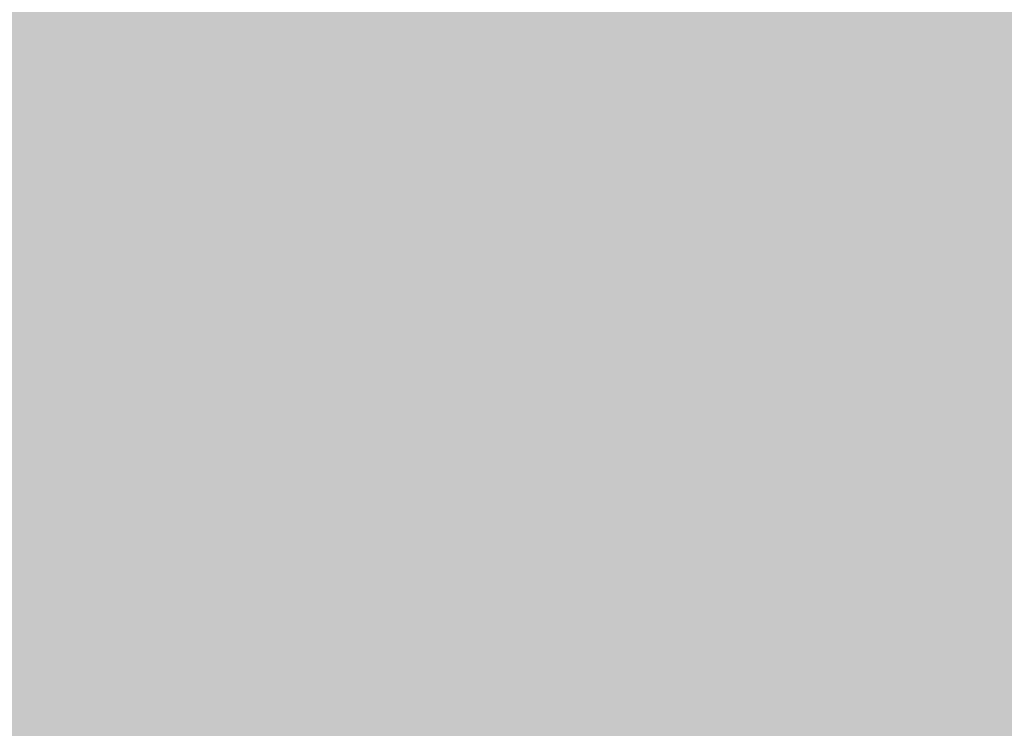
# Model space of a CAD drawing. Units: feet. Extents: x 3168 to 4724, y 827 to 1477.
# Tile 182 of 256: x 3307.378 to 3316.072, y 1087.401 to 1093.654. Entities that reach past the tile are written whole.
import ezdxf

# ---------------------------------------------------------------- set-up
doc = ezdxf.new("R2010")
doc.units = ezdxf.units.FT
doc.layers.add('A-ELEV-PATT', color=8, linetype='Continuous', lineweight=13)

msp = doc.modelspace()

# ---------------------------------------------------------------- hatches: boundary and pattern name
at = {"layer": 'A-ELEV-PATT'}
h = msp.add_hatch(color=256, dxfattribs=at)
h.dxf.hatch_style = 1
edge = h.paths.add_edge_path()
edge.add_ellipse((3552.9058, 979.2201), major_axis=(36.7449, 0), ratio=0.4848485, start_angle=0, end_angle=360)
edge = h.paths.add_edge_path()
edge.add_ellipse((3559.8916, 929.2523), major_axis=(36.7449, 0), ratio=0.4848485, start_angle=0, end_angle=360)
edge = h.paths.add_edge_path()
edge.add_line((3299.3168, 1198.6061), (3479.9167, 1198.6061))
edge.add_line((3479.9167, 1198.6061), (3479.9167, 1209.8686))
edge.add_spline(control_points=[(3479.9167, 1209.8686), (3464.3012, 1209.8686), (3448.6856, 1209.8686), (3410.9491, 1209.8686), (3388.8282, 1209.8686), (3355.6469, 1209.8686), (3344.5864, 1209.8686), (3327.9957, 1209.8686), (3322.4655, 1209.8686), (3314.1702, 1209.8686), (3311.4051, 1209.8686), (3307.2574, 1209.8686), (3305.8748, 1209.8686), (3303.801, 1209.8686), (3303.1097, 1209.8686), (3302.0728, 1209.8686), (3301.7272, 1209.8686), (3301.2087, 1209.8686), (3301.0359, 1209.8686), (3300.7767, 1209.8686), (3300.6903, 1209.8686), (3300.5606, 1209.8686), (3300.5174, 1209.8686), (3300.4526, 1209.8686), (3300.431, 1209.8686), (3300.3986, 1209.8686), (3300.3878, 1209.8686), (3300.3662, 1209.8686), (3300.3457, 1209.8686), (3300.3455, 1209.8686), (3300.3455, 1209.8686), (3300.3433, 1209.8686), (3300.3411, 1209.8686), (3300.3379, 1209.8686), (3300.3368, 1209.8686), (3300.3339, 1209.8686), (3300.3321, 1209.8686), (3300.3255, 1209.8686), (3300.3207, 1209.8686), (3300.3109, 1209.8686), (3300.306, 1209.8686), (3300.2905, 1209.8686), (3300.28, 1209.8686), (3300.2324, 1209.8688), (3300.1953, 1209.869), (3299.9511, 1209.8706), (3299.7448, 1209.8743), (3299.4368, 1209.8833), (3299.3344, 1209.8868), (3299.1811, 1209.8929), (3299.13, 1209.8951), (3298.6522, 1209.9168), (3298.2295, 1209.9457), (3297.6016, 1210.0024), (3297.3934, 1210.0235), (3297.0827, 1210.0583), (3296.9793, 1210.0705), (3296.293, 1210.1549), (3295.7181, 1210.2434), (3294.8687, 1210.3989), (3294.5877, 1210.4545), (3294.1693, 1210.5433), (3294.0304, 1210.5739), (3291.7071, 1211.1012), (3289.6536, 1211.8134), (3285.7763, 1213.564), (3283.9514, 1214.6035), (3280.5122, 1216.9801), (3278.8972, 1218.3176), (3276.3799, 1220.8295), (3275.416, 1221.9177), (3274.0393, 1223.7077), (3273.581, 1224.3495), (3273.1432, 1225.0163)], knot_values=[39.119033, 39.119033, 39.119033, 39.119033, 39.286353, 39.286353, 39.523379, 39.523379, 39.641892, 39.641892, 39.701148, 39.701148, 39.730777, 39.730777, 39.745591, 39.745591, 39.752998, 39.752998, 39.756701, 39.756701, 39.758553, 39.758553, 39.759479, 39.759479, 39.759942, 39.759942, 39.760173, 39.760173, 39.760289, 39.760289, 39.760405, 39.760405, 39.760463, 39.760463, 39.763389, 39.763389, 39.764851, 39.764851, 39.767304, 39.767304, 39.773825, 39.773825, 39.78057, 39.78057, 39.79477, 39.79477, 39.845194, 39.845194, 40.126715, 40.126715, 40.267476, 40.267476, 40.337856, 40.337856, 40.927023, 40.927023, 41.221606, 41.221606, 41.368898, 41.368898, 42.202622, 42.202622, 42.619485, 42.619485, 42.827916, 42.827916, 46.118323, 46.118323, 49.408731, 49.408731, 52.699139, 52.699139, 54.927489, 54.927489, 56.104228, 56.104228, 56.104228, 56.104228], weights=[1, 1, 1, 1, 1, 1, 1, 1, 1, 1, 1, 1, 1, 1, 1, 1, 1, 1, 1, 1, 1, 1, 1, 1, 1, 1, 1, 1, 1, 1, 1, 1, 1, 1, 1, 1, 1, 1, 1, 1, 1, 1, 1, 1, 1, 1, 1, 1, 1, 1, 1, 1, 1, 1, 1, 1, 1, 1, 1, 1, 1, 1, 1, 1, 1, 1, 1, 1, 1, 1, 1, 1, 1, 1], degree=3, periodic=0)
edge.add_line((3273.1432, 1225.0163), (3273.1432, 1099.0163))
edge.add_line((3273.1432, 1099.0163), (3299.3168, 1099.0163))
edge.add_line((3299.3168, 1099.0163), (3299.3168, 1198.6061))
edge = h.paths.add_edge_path()
edge.add_line((3304.7584, 1324.1581), (3479.9167, 1324.1581))
edge.add_line((3479.9167, 1324.1581), (3479.9167, 1335.7146))
edge.add_line((3479.9167, 1335.7146), (3269.1616, 1335.7146))
edge.add_spline(control_points=[(3269.1616, 1335.7146), (3264.0242, 1335.7146), (3258.3641, 1328.9582), (3259.2643, 1323.9003)], knot_values=[0, 0, 0, 0, 15.412191, 15.412191, 15.412191, 15.412191], degree=3, periodic=0)
edge.add_line((3259.2643, 1323.9003), (3265.5168, 1288.7691))
edge.add_line((3265.5168, 1288.7691), (3275.2651, 1261.5456))
edge.add_line((3275.2651, 1261.5456), (3304.7584, 1261.5456))
edge.add_line((3304.7584, 1261.5456), (3304.7584, 1324.1581))
h = msp.add_hatch(color=256, dxfattribs=at)
h.dxf.hatch_style = 1
h.paths.add_polyline_path([(3384.5252, 1099.0163), (3335.0292, 1099.0163), (3299.3168, 1099.0163), (3273.1432, 1099.0163), (3217.5654, 1099.0163), (3168.0693, 827.1163), (3335.0292, 827.1163)])

doc.saveas('drawing.dxf')
